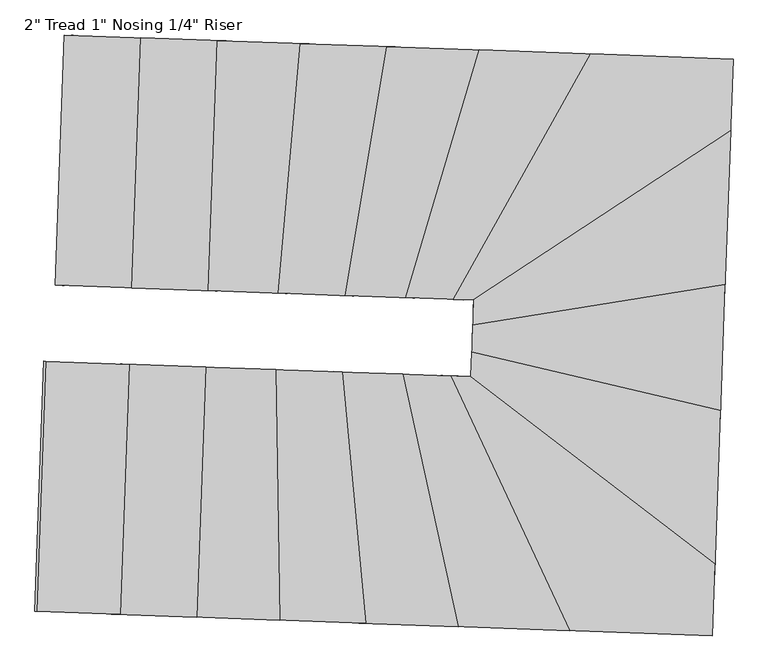
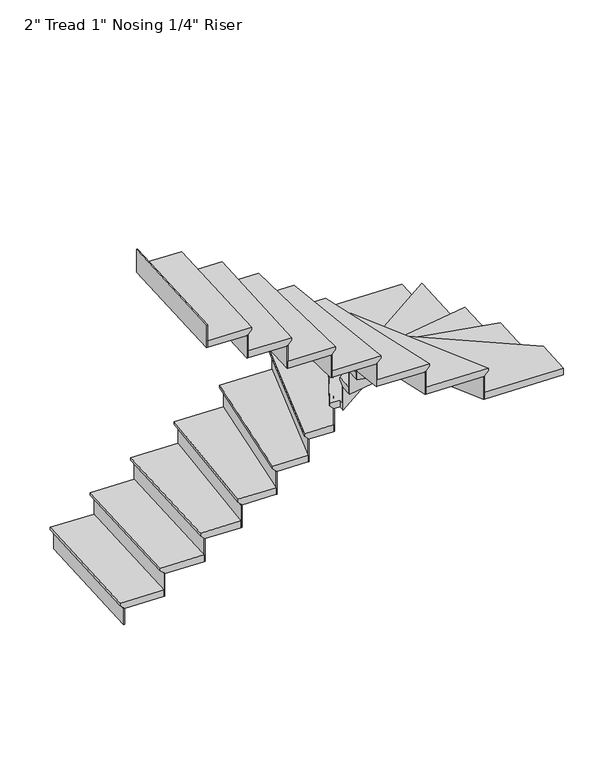
"""IFC4 building model written with IfcOpenShell, lengths in millimetres: stair flight geometry."""

from ifc_helpers import new_model, si_unit, origin, place, context, project, spatial, faceted_brep, source, transform, mapped, element, save


def stair_flight_55d3e88d(model_context):
    return source(origin(), model_context, "Body", "Brep", [
        faceted_brep([(-10039.2744432, -1277.1215258, 3198.2833333), (-10039.2744432, -1277.1215258, 3217.3333333), (-10006.394185, -363.3128759, 3217.3333333), (-10006.394185, -363.3128759, 3198.2833333), (-10013.8908696, -1278.0348663, 3172.8833333), (-9981.0106114, -364.2262164, 3172.8833333), (-9734.6715599, -1288.0816118, 3217.3333333), (-9701.7913017, -374.272962, 3217.3333333), (-9981.0106114, -364.2262164, 3166.5333333), (-9701.7913017, -374.272962, 3166.5333333), (-9734.6715599, -1288.0816118, 3166.5333333), (-10013.8908696, -1278.0348663, 3166.5333333)], [[[0, 1, 2, 3]], [[4, 0, 3, 5]], [[2, 1, 6, 7]], [[8, 9, 10, 11]], [[2, 7, 9, 8, 5, 3]], [[8, 11, 4, 5]], [[6, 1, 0, 4, 11, 10]], [[7, 6, 10, 9]]]),
        faceted_brep([(-10013.8908696, -1278.0348663, 3166.5333333), (-10013.8908696, -1278.0348663, 3048.0), (-10007.5449762, -1278.2632014, 3048.0), (-10007.5449762, -1278.2632014, 3166.5333333), (-9981.0106114, -364.2262164, 3166.5333333), (-9974.664718, -364.4545515, 3166.5333333), (-9974.664718, -364.4545515, 3048.0), (-9981.0106114, -364.2262164, 3048.0)], [[[0, 1, 2, 3]], [[4, 5, 6, 7]], [[1, 0, 4, 7]], [[2, 1, 7, 6]], [[3, 2, 6, 5]], [[0, 3, 5, 4]]]),
        faceted_brep([(-9734.6715599, -1288.0816118, 3335.8666667), (-9734.6715599, -1288.0816118, 3166.5333333), (-9728.3256665, -1288.309947, 3166.5333333), (-9728.3256665, -1288.309947, 3335.8666667), (-9701.7913017, -374.272962, 3335.8666667), (-9695.4454083, -374.5012971, 3335.8666667), (-9695.4454083, -374.5012971, 3166.5333333), (-9701.7913017, -374.272962, 3166.5333333)], [[[0, 1, 2, 3]], [[4, 5, 6, 7]], [[1, 0, 4, 7]], [[2, 1, 7, 6]], [[3, 2, 6, 5]], [[0, 3, 5, 4]]]),
        faceted_brep([(-9727.1748753, -373.3596215, 3386.6666667), (-9760.0551335, -1287.1682713, 3386.6666667), (-9455.4522502, -1298.1283574, 3386.6666667), (-9422.571992, -384.3197075, 3386.6666667), (-9701.7913017, -374.272962, 3335.8666667), (-9422.571992, -384.3197075, 3335.8666667), (-9455.4522502, -1298.1283574, 3335.8666667), (-9734.6715599, -1288.0816118, 3335.8666667), (-9701.7913017, -374.272962, 3342.2166667), (-9727.1748753, -373.3596215, 3367.6166667), (-9734.6715599, -1288.0816118, 3342.2166667), (-9760.0551335, -1287.1682713, 3367.6166667)], [[[0, 1, 2, 3]], [[4, 5, 6, 7]], [[0, 3, 5, 4, 8, 9]], [[4, 7, 10, 8]], [[2, 1, 11, 10, 7, 6]], [[3, 2, 6, 5]], [[11, 1, 0, 9]], [[10, 11, 9, 8]]]),
        faceted_brep([(-9455.4522502, -1298.1283574, 3505.2), (-9455.4522502, -1298.1283574, 3335.8666667), (-9449.1063568, -1298.3566925, 3335.8666667), (-9449.1063568, -1298.3566925, 3505.2), (-9422.571992, -384.3197075, 3505.2), (-9416.2260986, -384.5480426, 3505.2), (-9416.2260986, -384.5480426, 3335.8666667), (-9422.571992, -384.3197075, 3335.8666667)], [[[0, 1, 2, 3]], [[4, 5, 6, 7]], [[1, 0, 4, 7]], [[2, 1, 7, 6]], [[3, 2, 6, 5]], [[0, 3, 5, 4]]]),
        faceted_brep([(-9447.9555656, -383.406367, 3556.0), (-9480.8358238, -1297.2150169, 3556.0), (-9199.9504308, -1307.3217107, 3556.0), (-9119.566643, -395.2223118, 3556.0), (-9422.571992, -384.3197075, 3505.2), (-9119.566643, -395.2223118, 3505.2), (-9199.9504308, -1307.3217107, 3505.2), (-9455.4522502, -1298.1283574, 3505.2), (-9422.571992, -384.3197075, 3511.55), (-9447.9555656, -383.406367, 3536.95), (-9455.4522502, -1298.1283574, 3511.55), (-9480.8358238, -1297.2150169, 3536.95)], [[[0, 1, 2, 3]], [[4, 5, 6, 7]], [[0, 3, 5, 4, 8, 9]], [[4, 7, 10, 8]], [[2, 1, 11, 10, 7, 6]], [[3, 2, 6, 5]], [[11, 1, 0, 9]], [[10, 11, 9, 8]]]),
        faceted_brep([(-9199.9504308, -1307.3217107, 3674.5333333), (-9199.9504308, -1307.3217107, 3505.2), (-9193.5959688, -1307.5503542, 3505.2), (-9193.5959688, -1307.5503542, 3674.5333333), (-9119.566643, -395.2223118, 3674.5333333), (-9113.212181, -395.4509552, 3674.5333333), (-9113.212181, -395.4509552, 3505.2), (-9119.566643, -395.2223118, 3505.2)], [[[0, 1, 2, 3]], [[4, 5, 6, 7]], [[1, 0, 4, 7]], [[2, 1, 7, 6]], [[3, 2, 6, 5]], [[0, 3, 5, 4]]]),
        faceted_brep([(-9144.9844911, -394.3077381, 3725.3333333), (-9225.3682789, -1306.407137, 3725.3333333), (-8955.9416356, -1316.1015272, 3725.3333333), (-8804.7818676, -406.5487582, 3725.3333333), (-9119.566643, -395.2223118, 3674.5333333), (-8804.7818676, -406.5487582, 3674.5333333), (-8955.9416356, -1316.1015272, 3674.5333333), (-9199.9504308, -1307.3217107, 3674.5333333), (-9119.566643, -395.2223118, 3680.8833333), (-9144.9844911, -394.3077381, 3706.2833333), (-9199.9504308, -1307.3217107, 3680.8833333), (-9225.3682789, -1306.407137, 3706.2833333)], [[[0, 1, 2, 3]], [[4, 5, 6, 7]], [[0, 3, 5, 4, 8, 9]], [[4, 7, 10, 8]], [[2, 1, 11, 10, 7, 6]], [[3, 2, 6, 5]], [[11, 1, 0, 9]], [[10, 11, 9, 8]]]),
        faceted_brep([(-8955.9416356, -1316.1015272, 3843.8666667), (-8955.9416356, -1316.1015272, 3674.5333333), (-8949.5428047, -1316.3317671, 3674.5333333), (-8949.5428047, -1316.3317671, 3843.8666667), (-8804.7818676, -406.5487582, 3843.8666667), (-8798.3830367, -406.7789981, 3843.8666667), (-8798.3830367, -406.7789981, 3674.5333333), (-8804.7818676, -406.5487582, 3674.5333333)], [[[0, 1, 2, 3]], [[4, 5, 6, 7]], [[1, 0, 4, 7]], [[2, 1, 7, 6]], [[3, 2, 6, 5]], [[0, 3, 5, 4]]]),
        faceted_brep([(-8830.3771913, -405.6277986, 3894.6666667), (-8981.5369593, -1315.1805676, 3894.6666667), (-8734.4577413, -1324.0708626, 3894.6666667), (-8466.5990966, -418.7171009, 3894.6666667), (-8804.7818676, -406.5487582, 3843.8666667), (-8466.5990966, -418.7171009, 3843.8666667), (-8734.4577413, -1324.0708626, 3843.8666667), (-8955.9416356, -1316.1015272, 3843.8666667), (-8804.7818676, -406.5487582, 3850.2166667), (-8830.3771913, -405.6277986, 3875.6166667), (-8955.9416356, -1316.1015272, 3850.2166667), (-8981.5369593, -1315.1805676, 3875.6166667)], [[[0, 1, 2, 3]], [[4, 5, 6, 7]], [[0, 3, 5, 4, 8, 9]], [[4, 7, 10, 8]], [[2, 1, 11, 10, 7, 6]], [[3, 2, 6, 5]], [[11, 1, 0, 9]], [[10, 11, 9, 8]]]),
        faceted_brep([(-8734.4577413, -1324.0708626, 4013.2), (-8734.4577413, -1324.0708626, 3843.8666667), (-8727.9054047, -1324.3066258, 3843.8666667), (-8727.9054047, -1324.3066258, 4013.2), (-8466.5990966, -418.7171009, 4013.2), (-8460.0467599, -418.9528642, 4013.2), (-8460.0467599, -418.9528642, 3843.8666667), (-8466.5990966, -418.7171009, 3843.8666667)], [[[0, 1, 2, 3]], [[4, 5, 6, 7]], [[1, 0, 4, 7]], [[2, 1, 7, 6]], [[3, 2, 6, 5]], [[0, 3, 5, 4]]]),
        faceted_brep([(-8492.8084432, -417.7740478, 4064.0), (-8760.667088, -1323.1278095, 4064.0), (-8558.2251501, -1330.4119856, 4064.0), (-8056.8234634, -433.4614663, 4064.0), (-8466.5990966, -418.7171009, 4013.2), (-8056.8234634, -433.4614663, 4013.2), (-8558.2251501, -1330.4119856, 4013.2), (-8734.4577413, -1324.0708626, 4013.2), (-8466.5990966, -418.7171009, 4019.55), (-8492.8084432, -417.7740478, 4044.95), (-8734.4577413, -1324.0708626, 4019.55), (-8760.667088, -1323.1278095, 4044.95)], [[[0, 1, 2, 3]], [[4, 5, 6, 7]], [[0, 3, 5, 4, 8, 9]], [[4, 7, 10, 8]], [[2, 1, 11, 10, 7, 6]], [[3, 2, 6, 5]], [[11, 1, 0, 9]], [[10, 11, 9, 8]]]),
        faceted_brep([(-8558.2251501, -1330.4119856, 4182.5333333), (-8558.2251501, -1330.4119856, 4013.2), (-8551.0937819, -1330.6685834, 4013.2), (-8551.0937819, -1330.6685834, 4182.5333333), (-8056.8234634, -433.4614663, 4182.5333333), (-8049.6920951, -433.718064, 4182.5333333), (-8049.6920951, -433.718064, 4013.2), (-8056.8234634, -433.4614663, 4013.2)], [[[0, 1, 2, 3]], [[4, 5, 6, 7]], [[1, 0, 4, 7]], [[2, 1, 7, 6]], [[3, 2, 6, 5]], [[0, 3, 5, 4]]]),
        faceted_brep([(-7576.4021107, -744.6189573, 4233.3333333), (-7565.8418401, -451.1277497, 4233.3333333), (-8085.3489363, -432.4350754, 4233.3333333), (-8586.750623, -1329.3855947, 4233.3333333), (-8512.5307482, -1332.0561414, 4233.3333333), (-8513.5934983, -1361.5921107, 4233.3333333), (-7565.8418401, -451.1277497, 4182.5333333), (-7576.4021107, -744.6189573, 4182.5333333), (-8513.5934983, -1361.5921107, 4182.5333333), (-8512.5307482, -1332.0561414, 4182.5333333), (-8558.2251501, -1330.4119856, 4182.5333333), (-8056.8234634, -433.4614663, 4182.5333333), (-8056.8234634, -433.4614663, 4188.8833333), (-8085.3489363, -432.4350754, 4214.2833333), (-8558.2251501, -1330.4119856, 4188.8833333), (-8586.750623, -1329.3855947, 4214.2833333)], [[[0, 1, 2, 3, 4, 5]], [[6, 7, 8, 9, 10, 11]], [[1, 0, 7, 6]], [[2, 1, 6, 11, 12, 13]], [[11, 10, 14, 12]], [[4, 3, 15, 14, 10, 9]], [[5, 4, 9, 8]], [[0, 5, 8, 7]], [[15, 3, 2, 13]], [[14, 15, 13, 12]]]),
        faceted_brep([(-8513.5934983, -1361.5921107, 4351.8666667), (-8513.5934983, -1361.5921107, 4182.5333333), (-8513.8736844, -1369.3790464, 4182.5333333), (-8513.8736844, -1369.3790464, 4351.8666667), (-7576.4021107, -744.6189573, 4351.8666667), (-7576.6822968, -752.405893, 4351.8666667), (-7576.6822968, -752.405893, 4182.5333333), (-7576.4021107, -744.6189573, 4182.5333333)], [[[0, 1, 2, 3]], [[4, 5, 6, 7]], [[1, 0, 4, 7]], [[2, 1, 7, 6]], [[3, 2, 6, 5]], [[0, 3, 5, 4]]]),
        faceted_brep([(-7575.2813665, -713.4712147, 4402.6666667), (-8512.472754, -1330.4443681, 4402.6666667), (-8516.7022393, -1447.9902872, 4402.6666667), (-7596.4124368, -1300.7462523, 4402.6666667), (-7576.4021107, -744.6189573, 4351.8666667), (-7596.4124368, -1300.7462523, 4351.8666667), (-8516.7022393, -1447.9902872, 4351.8666667), (-8513.5934983, -1361.5921107, 4351.8666667), (-7576.4021107, -744.6189573, 4358.2166667), (-7575.2813665, -713.4712147, 4383.6166667), (-8513.5934983, -1361.5921107, 4358.2166667), (-8512.472754, -1330.4443681, 4383.6166667)], [[[0, 1, 2, 3]], [[4, 5, 6, 7]], [[0, 3, 5, 4, 8, 9]], [[4, 7, 10, 8]], [[2, 1, 11, 10, 7, 6]], [[3, 2, 6, 5]], [[11, 1, 0, 9]], [[10, 11, 9, 8]]]),
        faceted_brep([(-8516.7022393, -1447.9902872, 4521.2), (-8516.7022393, -1447.9902872, 4351.8666667), (-8516.934968, -1454.458287, 4351.8666667), (-8516.934968, -1454.458287, 4521.2), (-7596.4124368, -1300.7462523, 4521.2), (-7596.6451655, -1307.2142521, 4521.2), (-7596.6451655, -1307.2142521, 4351.8666667), (-7596.4124368, -1300.7462523, 4351.8666667)], [[[0, 1, 2, 3]], [[4, 5, 6, 7]], [[1, 0, 4, 7]], [[2, 1, 7, 6]], [[3, 2, 6, 5]], [[0, 3, 5, 4]]]),
        faceted_brep([(-7595.481522, -1274.874253, 4572.0), (-8515.7713244, -1422.1182879, 4572.0), (-8520.2678323, -1547.0853038, 4572.0), (-7612.9403349, -1760.0898551, 4572.0), (-7596.4124368, -1300.7462523, 4521.2), (-7612.9403349, -1760.0898551, 4521.2), (-8520.2678323, -1547.0853038, 4521.2), (-8516.7022393, -1447.9902872, 4521.2), (-7596.4124368, -1300.7462523, 4527.55), (-7595.481522, -1274.874253, 4552.95), (-8516.7022393, -1447.9902872, 4527.55), (-8515.7713244, -1422.1182879, 4552.95)], [[[0, 1, 2, 3]], [[4, 5, 6, 7]], [[0, 3, 5, 4, 8, 9]], [[4, 7, 10, 8]], [[2, 1, 11, 10, 7, 6]], [[3, 2, 6, 5]], [[11, 1, 0, 9]], [[10, 11, 9, 8]]]),
        faceted_brep([(-8520.2678323, -1547.0853038, 4690.5333333), (-8520.2678323, -1547.0853038, 4521.2), (-8520.500561, -1553.5533036, 4521.2), (-8520.500561, -1553.5533036, 4690.5333333), (-7612.9403349, -1760.0898551, 4690.5333333), (-7613.1730636, -1766.5578549, 4690.5333333), (-7613.1730636, -1766.5578549, 4521.2), (-7612.9403349, -1760.0898551, 4521.2)], [[[0, 1, 2, 3]], [[4, 5, 6, 7]], [[1, 0, 4, 7]], [[2, 1, 7, 6]], [[3, 2, 6, 5]], [[0, 3, 5, 4]]]),
        faceted_brep([(-7612.0094201, -1734.2178558, 4741.3333333), (-8519.3369174, -1521.2133045, 4741.3333333), (-8522.5774937, -1611.2754511, 4741.3333333), (-8568.6431579, -1609.6179367, 4741.3333333), (-7633.3303199, -2326.7686368, 4741.3333333), (-7612.9403349, -1760.0898551, 4690.5333333), (-7633.3303199, -2326.7686368, 4690.5333333), (-8568.6431579, -1609.6179367, 4690.5333333), (-8522.5774937, -1611.2754511, 4690.5333333), (-8520.2678323, -1547.0853038, 4690.5333333), (-7612.9403349, -1760.0898551, 4696.8833333), (-7612.0094201, -1734.2178558, 4722.2833333), (-8520.2678323, -1547.0853038, 4696.8833333), (-8519.3369174, -1521.2133045, 4722.2833333)], [[[0, 1, 2, 3, 4]], [[5, 6, 7, 8, 9]], [[0, 4, 6, 5, 10, 11]], [[5, 9, 12, 10]], [[2, 1, 13, 12, 9, 8]], [[3, 2, 8, 7]], [[4, 3, 7, 6]], [[13, 1, 0, 11]], [[12, 13, 11, 10]]]),
        faceted_brep([(-8568.6431579, -1609.6179367, 4859.8666667), (-8568.6431579, -1609.6179367, 4690.5333333), (-8579.5929645, -1609.2239456, 4690.5333333), (-8579.5929645, -1609.2239456, 4859.8666667), (-7633.3303199, -2326.7686368, 4859.8666667), (-7633.610506, -2334.5555724, 4859.8666667), (-7633.610506, -2334.5555724, 4690.5333333), (-7633.3303199, -2326.7686368, 4690.5333333)], [[[0, 1, 2, 3]], [[4, 5, 6, 7]], [[1, 0, 4, 7]], [[2, 1, 7, 6]], [[3, 2, 6, 5]], [[0, 3, 5, 4]]]),
        faceted_brep([(-8189.6816712, -2538.2452939, 4910.6666667), (-7641.649102, -2557.9643591, 4910.6666667), (-7632.2095756, -2295.6208941, 4910.6666667), (-8524.8439316, -1611.1939011, 4910.6666667), (-8625.3228415, -1607.5785134, 4910.6666667), (-7641.649102, -2557.9643591, 4859.8666667), (-8189.6816712, -2538.2452939, 4859.8666667), (-8625.3228415, -1607.5785134, 4859.8666667), (-8568.6431579, -1609.6179367, 4859.8666667), (-7633.3303199, -2326.7686368, 4859.8666667), (-7633.3303199, -2326.7686368, 4866.2166667), (-7632.2095756, -2295.6208941, 4891.6166667), (-8568.6431579, -1609.6179367, 4866.2166667), (-8524.8439316, -1611.1939011, 4891.6166667)], [[[0, 1, 2, 3, 4]], [[5, 6, 7, 8, 9]], [[1, 0, 6, 5]], [[2, 1, 5, 9, 10, 11]], [[9, 8, 12, 10]], [[4, 3, 13, 12, 8, 7]], [[0, 4, 7, 6]], [[13, 3, 2, 11]], [[12, 13, 11, 10]]]),
        faceted_brep([(-8625.3228415, -1607.5785134, 5029.2), (-8625.3228415, -1607.5785134, 4859.8666667), (-8632.4542098, -1607.3219157, 4859.8666667), (-8632.4542098, -1607.3219157, 5029.2), (-8189.6816712, -2538.2452939, 5029.2), (-8196.8130394, -2537.9886962, 5029.2), (-8196.8130394, -2537.9886962, 4859.8666667), (-8189.6816712, -2538.2452939, 4859.8666667)], [[[0, 1, 2, 3]], [[4, 5, 6, 7]], [[1, 0, 4, 7]], [[2, 1, 7, 6]], [[3, 2, 6, 5]], [[0, 3, 5, 4]]]),
        faceted_brep([(-8161.1561983, -2539.2716849, 5080.0), (-8596.7973686, -1608.6049044, 5080.0), (-8796.9231803, -1601.404066, 5080.0), (-8594.8250519, -2523.6676042, 5080.0), (-8189.6816712, -2538.2452939, 5029.2), (-8594.8250519, -2523.6676042, 5029.2), (-8796.9231803, -1601.404066, 5029.2), (-8625.3228415, -1607.5785134, 5029.2), (-8189.6816712, -2538.2452939, 5035.55), (-8161.1561983, -2539.2716849, 5060.95), (-8625.3228415, -1607.5785134, 5035.55), (-8596.7973686, -1608.6049044, 5060.95)], [[[0, 1, 2, 3]], [[4, 5, 6, 7]], [[0, 3, 5, 4, 8, 9]], [[4, 7, 10, 8]], [[2, 1, 11, 10, 7, 6]], [[3, 2, 6, 5]], [[11, 1, 0, 9]], [[10, 11, 9, 8]]]),
        faceted_brep([(-8796.9231803, -1601.404066, 5198.5333333), (-8796.9231803, -1601.404066, 5029.2), (-8803.475517, -1601.1683028, 5029.2), (-8803.475517, -1601.1683028, 5198.5333333), (-8594.8250519, -2523.6676042, 5198.5333333), (-8601.3773886, -2523.4318409, 5198.5333333), (-8601.3773886, -2523.4318409, 5029.2), (-8594.8250519, -2523.6676042, 5029.2)], [[[0, 1, 2, 3]], [[4, 5, 6, 7]], [[1, 0, 4, 7]], [[2, 1, 7, 6]], [[3, 2, 6, 5]], [[0, 3, 5, 4]]]),
        faceted_brep([(-8568.6157052, -2524.6106573, 5249.3333333), (-8770.7138336, -1602.3471191, 5249.3333333), (-9017.1790286, -1593.4789176, 5249.3333333), (-8931.779777, -2511.5434485, 5249.3333333), (-8594.8250519, -2523.6676042, 5198.5333333), (-8931.779777, -2511.5434485, 5198.5333333), (-9017.1790286, -1593.4789176, 5198.5333333), (-8796.9231803, -1601.404066, 5198.5333333), (-8594.8250519, -2523.6676042, 5204.8833333), (-8568.6157052, -2524.6106573, 5230.2833333), (-8796.9231803, -1601.404066, 5204.8833333), (-8770.7138336, -1602.3471191, 5230.2833333)], [[[0, 1, 2, 3]], [[4, 5, 6, 7]], [[0, 3, 5, 4, 8, 9]], [[4, 7, 10, 8]], [[2, 1, 11, 10, 7, 6]], [[3, 2, 6, 5]], [[11, 1, 0, 9]], [[10, 11, 9, 8]]]),
        faceted_brep([(-9017.1790286, -1593.4789176, 5367.8666667), (-9017.1790286, -1593.4789176, 5198.5333333), (-9023.5778595, -1593.2486777, 5198.5333333), (-9023.5778595, -1593.2486777, 5367.8666667), (-8931.779777, -2511.5434485, 5367.8666667), (-8938.1786079, -2511.3132086, 5367.8666667), (-8938.1786079, -2511.3132086, 5198.5333333), (-8931.779777, -2511.5434485, 5198.5333333)], [[[0, 1, 2, 3]], [[4, 5, 6, 7]], [[1, 0, 4, 7]], [[2, 1, 7, 6]], [[3, 2, 6, 5]], [[0, 3, 5, 4]]]),
        faceted_brep([(-8906.1844533, -2512.4644081, 5418.6666667), (-8991.5837049, -1594.3998772, 5418.6666667), (-9260.8328726, -1584.7118729, 5418.6666667), (-9246.2096012, -2500.2297738, 5418.6666667), (-8931.779777, -2511.5434485, 5367.8666667), (-9246.2096012, -2500.2297738, 5367.8666667), (-9260.8328726, -1584.7118729, 5367.8666667), (-9017.1790286, -1593.4789176, 5367.8666667), (-8931.779777, -2511.5434485, 5374.2166667), (-8906.1844533, -2512.4644081, 5399.6166667), (-9017.1790286, -1593.4789176, 5374.2166667), (-8991.5837049, -1594.3998772, 5399.6166667)], [[[0, 1, 2, 3]], [[4, 5, 6, 7]], [[0, 3, 5, 4, 8, 9]], [[4, 7, 10, 8]], [[2, 1, 11, 10, 7, 6]], [[3, 2, 6, 5]], [[11, 1, 0, 9]], [[10, 11, 9, 8]]]),
        faceted_brep([(-9260.8328726, -1584.7118729, 5537.2), (-9260.8328726, -1584.7118729, 5367.8666667), (-9267.1873346, -1584.4832295, 5367.8666667), (-9267.1873346, -1584.4832295, 5537.2), (-9246.2096012, -2500.2297738, 5537.2), (-9252.5640632, -2500.0011303, 5537.2), (-9252.5640632, -2500.0011303, 5367.8666667), (-9246.2096012, -2500.2297738, 5367.8666667)], [[[0, 1, 2, 3]], [[4, 5, 6, 7]], [[1, 0, 4, 7]], [[2, 1, 7, 6]], [[3, 2, 6, 5]], [[0, 3, 5, 4]]]),
        faceted_brep([(-9220.7917531, -2501.1443475, 5588.0), (-9235.4150245, -1585.6264467, 5588.0), (-9516.266143, -1575.5209861, 5588.0), (-9549.1464012, -2489.329636, 5588.0), (-9246.2096012, -2500.2297738, 5537.2), (-9549.1464012, -2489.329636, 5537.2), (-9516.266143, -1575.5209861, 5537.2), (-9260.8328726, -1584.7118729, 5537.2), (-9246.2096012, -2500.2297738, 5543.55), (-9220.7917531, -2501.1443475, 5568.95), (-9260.8328726, -1584.7118729, 5543.55), (-9235.4150245, -1585.6264467, 5568.95)], [[[0, 1, 2, 3]], [[4, 5, 6, 7]], [[0, 3, 5, 4, 8, 9]], [[4, 7, 10, 8]], [[2, 1, 11, 10, 7, 6]], [[3, 2, 6, 5]], [[11, 1, 0, 9]], [[10, 11, 9, 8]]]),
        faceted_brep([(-9516.266143, -1575.5209861, 5706.5333333), (-9516.266143, -1575.5209861, 5537.2), (-9522.6120364, -1575.292651, 5537.2), (-9522.6120364, -1575.292651, 5706.5333333), (-9549.1464012, -2489.329636, 5706.5333333), (-9555.4922946, -2489.1013009, 5706.5333333), (-9555.4922946, -2489.1013009, 5537.2), (-9549.1464012, -2489.329636, 5537.2)], [[[0, 1, 2, 3]], [[4, 5, 6, 7]], [[1, 0, 4, 7]], [[2, 1, 7, 6]], [[3, 2, 6, 5]], [[0, 3, 5, 4]]]),
        faceted_brep([(-9523.7628276, -2490.2429765, 5757.3333333), (-9490.8825694, -1576.4343266, 5757.3333333), (-9795.4854527, -1565.4742405, 5757.3333333), (-9828.3657109, -2479.2828904, 5757.3333333), (-9549.1464012, -2489.329636, 5706.5333333), (-9828.3657109, -2479.2828904, 5706.5333333), (-9795.4854527, -1565.4742405, 5706.5333333), (-9516.266143, -1575.5209861, 5706.5333333), (-9549.1464012, -2489.329636, 5712.8833333), (-9523.7628276, -2490.2429765, 5738.2833333), (-9516.266143, -1575.5209861, 5712.8833333), (-9490.8825694, -1576.4343266, 5738.2833333)], [[[0, 1, 2, 3]], [[4, 5, 6, 7]], [[0, 3, 5, 4, 8, 9]], [[4, 7, 10, 8]], [[2, 1, 11, 10, 7, 6]], [[3, 2, 6, 5]], [[11, 1, 0, 9]], [[10, 11, 9, 8]]]),
        faceted_brep([(-9795.4854527, -1565.4742405, 5875.8666667), (-9795.4854527, -1565.4742405, 5706.5333333), (-9801.8313461, -1565.2459054, 5706.5333333), (-9801.8313461, -1565.2459054, 5875.8666667), (-9828.3657109, -2479.2828904, 5875.8666667), (-9834.7116043, -2479.0545553, 5875.8666667), (-9834.7116043, -2479.0545553, 5706.5333333), (-9828.3657109, -2479.2828904, 5706.5333333)], [[[0, 1, 2, 3]], [[4, 5, 6, 7]], [[1, 0, 4, 7]], [[2, 1, 7, 6]], [[3, 2, 6, 5]], [[0, 3, 5, 4]]]),
        faceted_brep([(-10074.7047624, -1555.427495, 6045.2), (-10074.7047624, -1555.427495, 5875.8666667), (-10081.0506558, -1555.1991598, 5875.8666667), (-10081.0506558, -1555.1991598, 6045.2), (-10107.5850206, -2469.2361449, 6045.2), (-10113.930914, -2469.0078097, 6045.2), (-10113.930914, -2469.0078097, 5875.8666667), (-10107.5850206, -2469.2361449, 5875.8666667)], [[[0, 1, 2, 3]], [[4, 5, 6, 7]], [[1, 0, 4, 7]], [[2, 1, 7, 6]], [[3, 2, 6, 5]], [[0, 3, 5, 4]]]),
        faceted_brep([(-9802.9821373, -2480.1962309, 5926.6666667), (-9770.1018791, -1566.387581, 5926.6666667), (-10074.7047624, -1555.427495, 5926.6666667), (-10107.5850206, -2469.2361449, 5926.6666667), (-9828.3657109, -2479.2828904, 5875.8666667), (-10107.5850206, -2469.2361449, 5875.8666667), (-10074.7047624, -1555.427495, 5875.8666667), (-9795.4854527, -1565.4742405, 5875.8666667), (-9828.3657109, -2479.2828904, 5882.2166667), (-9802.9821373, -2480.1962309, 5907.6166667), (-9795.4854527, -1565.4742405, 5882.2166667), (-9770.1018791, -1566.387581, 5907.6166667)], [[[0, 1, 2, 3]], [[4, 5, 6, 7]], [[0, 3, 5, 4, 8, 9]], [[4, 7, 10, 8]], [[2, 1, 11, 10, 7, 6]], [[3, 2, 6, 5]], [[11, 1, 0, 9]], [[10, 11, 9, 8]]]),
    ])


if __name__ == "__main__":
    model = new_model("IFC4")
    model_context = context("Model", 3, world=origin())
    ifc_project = project(units=[si_unit("LENGTHUNIT", "METRE", prefix="MILLI")], contexts=[model_context])
    site = spatial("IfcSite", under=ifc_project)
    building = spatial("IfcBuilding", under=site)
    placement = place(None, origin())
    stair_flight_shape = stair_flight_55d3e88d(model_context)
    element("IfcStairFlight", 1, ObjectType="2\" Tread 1\" Nosing 1/4\" Riser", at=placement, inside=building, context=model_context, shape_type="MappedRepresentation", body=[
        mapped(stair_flight_shape, transform((0.0, 0.0, 0.0), x_axis=(1.0, 0.0, 0.0), y_axis=(0.0, 1.0, 0.0), z_axis=(0.0, 0.0, 1.0))),
    ])
    save(model, "model.ifc")
